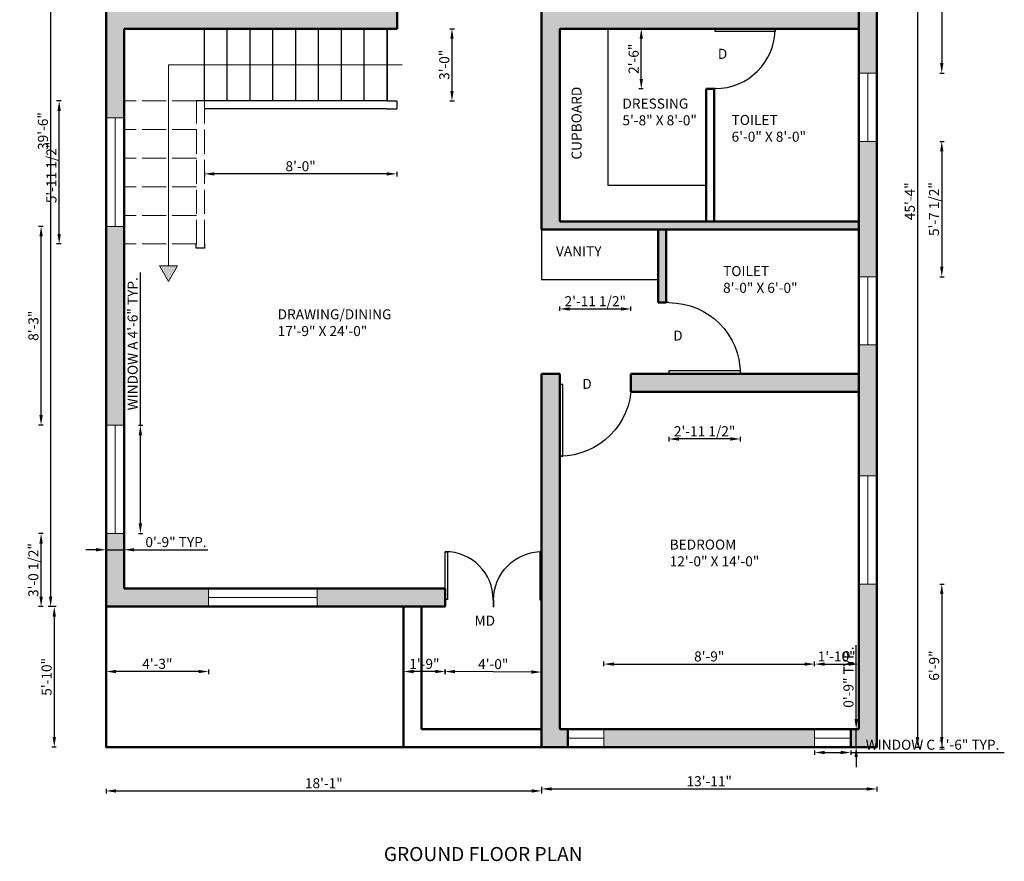
# Model space of a CAD drawing. Units: inches. Extents: x -41 to 449, y -587 to 56.
# Tile 1 of 2: x -41 to 449, y -587 to -167. Entities that reach past the tile are written whole.
import ezdxf

# ---------------------------------------------------------------- set-up
doc = ezdxf.new("R2010")
doc.units = ezdxf.units.IN
doc.linetypes.add('ACAD_ISO02W100', pattern=[15, 12, -3])
for name, color, linetype, lineweight in [('A-ANNO-DIMS', 2, 'Continuous', 18), ('A-ANNO-SYMB', 7, 'Continuous', 18), ('A-ANNO-TEXT', 7, 'Continuous', 18), ('A-ANNO-TITL', 7, 'Continuous', 35), ('A-AREA-IDEN', 7, 'Continuous', 25), ('A-DOOR', 3, 'Continuous', 25), ('A-FLOR-CASE', 8, 'Continuous', 25), ('A-FLOR-STRS', 7, 'Continuous', 25), ('A-FLOR-STRS-OVHD', 8, 'ACAD_ISO02W100', 18), ('A-GLAZ', 4, 'Continuous', 18), ('A-WALL', 7, 'Continuous', 50), ('A-WALL-PATT', 252, 'Continuous', 13)]:
    doc.layers.add(name, color=color, linetype=linetype, lineweight=lineweight)
doc.styles.get("Standard").update_dxf_attribs({"font": 'arial.ttf'})
doc.dimstyles.new('ISO-25', dxfattribs={"dimtxt": 5, "dimasz": 5, "dimexe": 1.25, "dimexo": 0.625, "dimtad": 1, "dimlunit": 3, "dimtxsty": 'Standard', "dimcen": 2.5, "dimadec": 0, "dimazin": 0, "dimtfac": 1, "dimtmove": 0, "dimatfit": 3, "dimfxl": 1, "dimfxlon": 1, "dimarcsym": 0})

# ---------------------------------------------------------------- blocks, each defined once
blk = doc.blocks.new('*U2')
for p, q in [((0, 0), (0, -6)), ((40, 0), (40, -6))]:
    blk.add_line(p, q)
blk.add_lwpolyline([(0, 0), (0, 40), (1.75, 40), (1.75, 0)], close=True)
blk.add_arc((0, 0), 40, 0, 90)
blk = doc.blocks.new('*D4')
at = {"layer": 'A-ANNO-DIMS', "color": 0, "lineweight": -2, "transparency": 16777216}
for p, q in [((404.95, 14.17), (407.2, 14.17)), ((405.95, 9.17), (405.95, -524.83)), ((404.95, -529.83), (407.2, -529.83))]:
    blk.add_line(p, q, dxfattribs=at)
at = {"layer": 'A-ANNO-DIMS', "color": 0, "transparency": 16777216}
for points in [[(405.11, 9.17), (406.78, 9.17), (405.95, 14.17)], [(405.11, -524.83), (406.78, -524.83), (405.95, -529.83)]]:
    blk.add_solid(points, dxfattribs=at)
at = {"layer": 'Defpoints', "color": 0, "transparency": 16777216}
for p in [(385.69, 14.17), (385.69, -529.83), (405.95, -529.83)]:
    blk.add_point(p, dxfattribs=at)
at = {"layer": 'A-ANNO-DIMS', "color": 0, "transparency": 16777216, "insert": (402.78, -257.83), "char_height": 5, "attachment_point": 5, "rotation": 90}
blk.add_mtext('45\'-4"', dxfattribs=at)
blk = doc.blocks.new('*D5')
at = {"layer": 'A-ANNO-DIMS', "color": 0, "lineweight": -2, "transparency": 16777216}
for p, q in [((-24.91, 14.17), (-27.16, 14.17)), ((-25.91, 9.17), (-25.91, -454.83)), ((-24.91, -459.83), (-27.16, -459.83))]:
    blk.add_line(p, q, dxfattribs=at)
at = {"layer": 'A-ANNO-DIMS', "color": 0, "transparency": 16777216}
for points in [[(-26.74, 9.17), (-25.07, 9.17), (-25.91, 14.17)], [(-26.74, -454.83), (-25.07, -454.83), (-25.91, -459.83)]]:
    blk.add_solid(points, dxfattribs=at)
at = {"layer": 'Defpoints', "color": 0, "transparency": 16777216}
for p in [(1.69, 14.17), (-25.91, -459.83), (1.69, -459.83)]:
    blk.add_point(p, dxfattribs=at)
at = {"layer": 'A-ANNO-DIMS', "color": 0, "transparency": 16777216, "insert": (-29.09, -222.83), "char_height": 5, "attachment_point": 5, "rotation": 90}
blk.add_mtext('39\'-6"', dxfattribs=at)
blk = doc.blocks.new('*D6')
at = {"layer": 'A-ANNO-DIMS', "color": 0, "lineweight": -2, "transparency": 16777216}
for p, q in [((-23.09, -459.83), (-25.34, -459.83)), ((-24.09, -464.83), (-24.09, -524.83)), ((-23.09, -529.83), (-25.34, -529.83))]:
    blk.add_line(p, q, dxfattribs=at)
at = {"layer": 'A-ANNO-DIMS', "color": 0, "transparency": 16777216}
for points in [[(-24.93, -464.83), (-23.26, -464.83), (-24.09, -459.83)], [(-24.93, -524.83), (-23.26, -524.83), (-24.09, -529.83)]]:
    blk.add_solid(points, dxfattribs=at)
at = {"layer": 'Defpoints', "color": 0, "transparency": 16777216}
for p in [(1.69, -459.83), (-24.09, -529.83), (1.69, -529.83)]:
    blk.add_point(p, dxfattribs=at)
at = {"layer": 'A-ANNO-DIMS', "color": 0, "transparency": 16777216, "insert": (-27.27, -494.83), "char_height": 5, "attachment_point": 5, "rotation": 90}
blk.add_mtext('5\'-10"', dxfattribs=at)
blk = doc.blocks.new('*D7')
at = {"layer": 'A-ANNO-DIMS', "color": 0, "lineweight": -2, "transparency": 16777216}
for p, q in [((1.69, -550.69), (1.69, -552.94)), ((6.69, -551.69), (213.69, -551.69)), ((218.69, -550.69), (218.69, -552.94))]:
    blk.add_line(p, q, dxfattribs=at)
at = {"layer": 'A-ANNO-DIMS', "color": 0, "transparency": 16777216}
for points in [[(6.69, -550.86), (6.69, -552.52), (1.69, -551.69)], [(213.69, -550.86), (213.69, -552.52), (218.69, -551.69)]]:
    blk.add_solid(points, dxfattribs=at)
at = {"layer": 'Defpoints', "color": 0, "transparency": 16777216}
for p in [(1.69, -529.83), (218.69, -529.83), (218.69, -551.69)]:
    blk.add_point(p, dxfattribs=at)
at = {"layer": 'A-ANNO-DIMS', "color": 0, "transparency": 16777216, "insert": (110.19, -548.51), "char_height": 5, "attachment_point": 5}
blk.add_mtext('18\'-1"', dxfattribs=at)
blk = doc.blocks.new('*D8')
at = {"layer": 'A-ANNO-DIMS', "color": 0, "lineweight": -2, "transparency": 16777216}
for p, q in [((218.69, -549.7), (218.69, -551.95)), ((223.69, -550.7), (380.69, -550.7)), ((385.69, -549.7), (385.69, -551.95))]:
    blk.add_line(p, q, dxfattribs=at)
at = {"layer": 'A-ANNO-DIMS', "color": 0, "transparency": 16777216}
for points in [[(223.69, -549.87), (223.69, -551.54), (218.69, -550.7)], [(380.69, -549.87), (380.69, -551.54), (385.69, -550.7)]]:
    blk.add_solid(points, dxfattribs=at)
at = {"layer": 'Defpoints', "color": 0, "transparency": 16777216}
for p in [(218.69, -529.83), (385.69, -529.83), (385.69, -550.7)]:
    blk.add_point(p, dxfattribs=at)
at = {"layer": 'A-ANNO-DIMS', "color": 0, "transparency": 16777216, "insert": (302.19, -547.52), "char_height": 5, "attachment_point": 5}
blk.add_mtext('13\'-11"', dxfattribs=at)
blk = doc.blocks.new('WIN-54IN')
blk.add_line((4.5, 54), (4.5, 0))
blk.add_lwpolyline([(0, 54), (9, 54), (9, 0), (0, 0)], close=True)
blk = doc.blocks.new('WIN-34IN')
blk.add_line((0, 4.5), (34, 4.5))
blk.add_lwpolyline([(0, 9), (34, 9), (34, 0), (0, 0)], close=True)
blk = doc.blocks.new('WIN-18IN')
blk.add_line((0, 4.5), (18, 4.5))
blk.add_lwpolyline([(0, 9), (18, 9), (18, 0), (0, 0)], close=True)
blk = doc.blocks.new('*D12')
at = {"layer": 'A-ANNO-DIMS', "color": 0, "lineweight": -2, "transparency": 16777216}
for p, q in [((18.79, -369.4), (18.79, -293.28)), ((17.79, -369.4), (20.04, -369.4)), ((18.79, -418.4), (18.79, -374.4)), ((17.79, -423.4), (20.04, -423.4))]:
    blk.add_line(p, q, dxfattribs=at)
at = {"layer": 'A-ANNO-DIMS', "color": 0, "transparency": 16777216}
for points in [[(17.96, -374.4), (19.63, -374.4), (18.79, -369.4)], [(17.96, -418.4), (19.63, -418.4), (18.79, -423.4)]]:
    blk.add_solid(points, dxfattribs=at)
at = {"layer": 'Defpoints', "color": 0, "transparency": 16777216}
for p in [(10.69, -369.4), (18.79, -369.4), (10.69, -423.4)]:
    blk.add_point(p, dxfattribs=at)
at = {"layer": 'A-ANNO-DIMS', "color": 0, "transparency": 16777216, "insert": (15.58, -328.84), "char_height": 5, "attachment_point": 5, "rotation": 90}
blk.add_mtext('WINDOW A 4\'-6" TYP.', dxfattribs=at)
blk = doc.blocks.new('*D13')
at = {"layer": 'A-ANNO-DIMS', "color": 0, "lineweight": -2, "transparency": 16777216}
for p, q in [((-3.31, -431.5), (-8.31, -431.5)), ((1.69, -430.5), (1.69, -432.75)), ((1.69, -431.5), (10.69, -431.5)), ((10.69, -430.5), (10.69, -432.75)), ((15.69, -431.5), (52.42, -431.5))]:
    blk.add_line(p, q, dxfattribs=at)
at = {"layer": 'A-ANNO-DIMS', "color": 0, "transparency": 16777216}
for points in [[(-3.31, -430.66), (-3.31, -432.33), (1.69, -431.5)], [(15.69, -430.66), (15.69, -432.33), (10.69, -431.5)]]:
    blk.add_solid(points, dxfattribs=at)
at = {"layer": 'Defpoints', "color": 0, "transparency": 16777216}
for p in [(1.69, -423.4), (10.69, -423.4), (10.69, -431.5)]:
    blk.add_point(p, dxfattribs=at)
at = {"layer": 'A-ANNO-DIMS', "color": 0, "transparency": 16777216, "insert": (36.56, -428.32), "char_height": 5, "attachment_point": 5}
blk.add_mtext('0\'-9" TYP.', dxfattribs=at)
blk = doc.blocks.new('*D16')
at = {"layer": 'A-ANNO-DIMS', "color": 0, "lineweight": -2, "transparency": 16777216}
for p, q in [((354.69, -531.53), (354.69, -533.78)), ((359.69, -532.53), (367.69, -532.53)), ((372.69, -531.53), (372.69, -533.78)), ((372.69, -532.53), (449.2, -532.53))]:
    blk.add_line(p, q, dxfattribs=at)
at = {"layer": 'A-ANNO-DIMS', "color": 0, "transparency": 16777216}
for points in [[(359.69, -531.7), (359.69, -533.37), (354.69, -532.53)], [(367.69, -531.7), (367.69, -533.37), (372.69, -532.53)]]:
    blk.add_solid(points, dxfattribs=at)
at = {"layer": 'Defpoints', "color": 0, "transparency": 16777216}
for p in [(354.69, -529.83), (372.69, -529.83), (372.69, -532.53)]:
    blk.add_point(p, dxfattribs=at)
at = {"layer": 'A-ANNO-DIMS', "color": 0, "transparency": 16777216, "insert": (413.45, -529.32), "char_height": 5, "attachment_point": 5}
blk.add_mtext('WINDOW C 1\'-6" TYP.', dxfattribs=at)
blk = doc.blocks.new('*D17')
at = {"layer": 'A-ANNO-DIMS', "color": 0, "lineweight": -2, "transparency": 16777216}
for p, q in [((375.39, -515.83), (375.39, -479.11)), ((374.39, -520.83), (376.64, -520.83)), ((375.39, -529.83), (375.39, -520.83)), ((374.39, -529.83), (376.64, -529.83)), ((375.39, -534.83), (375.39, -539.83))]:
    blk.add_line(p, q, dxfattribs=at)
at = {"layer": 'A-ANNO-DIMS', "color": 0, "transparency": 16777216}
for points in [[(374.56, -515.83), (376.23, -515.83), (375.39, -520.83)], [(374.56, -534.83), (376.23, -534.83), (375.39, -529.83)]]:
    blk.add_solid(points, dxfattribs=at)
at = {"layer": 'Defpoints', "color": 0, "transparency": 16777216}
for p in [(372.69, -520.83), (375.39, -520.83), (372.69, -529.83)]:
    blk.add_point(p, dxfattribs=at)
at = {"layer": 'A-ANNO-DIMS', "color": 0, "transparency": 16777216, "insert": (372.22, -494.97), "char_height": 5, "attachment_point": 5, "rotation": 90}
blk.add_mtext('0\'-9" TYP.', dxfattribs=at)
blk = doc.blocks.new('*D25')
at = {"layer": 'A-ANNO-DIMS', "color": 0, "lineweight": -2, "transparency": 16777216}
for p, q in [((417.04, -116.12), (419.29, -116.12)), ((418.04, -121.12), (418.04, -189)), ((417.04, -194), (419.29, -194))]:
    blk.add_line(p, q, dxfattribs=at)
at = {"layer": 'A-ANNO-DIMS', "color": 0, "transparency": 16777216}
for points in [[(417.21, -121.12), (418.88, -121.12), (418.04, -116.12)], [(417.21, -189), (418.88, -189), (418.04, -194)]]:
    blk.add_solid(points, dxfattribs=at)
at = {"layer": 'Defpoints', "color": 0, "transparency": 16777216}
for p in [(385.69, -116.12), (385.69, -194), (418.04, -194)]:
    blk.add_point(p, dxfattribs=at)
at = {"layer": 'A-ANNO-DIMS', "color": 0, "transparency": 16777216, "insert": (414.87, -155.06), "char_height": 5, "attachment_point": 5, "rotation": 90}
blk.add_mtext('6\'-6"', dxfattribs=at)
blk = doc.blocks.new('*D26')
at = {"layer": 'A-ANNO-DIMS', "color": 0, "lineweight": -2, "transparency": 16777216}
for p, q in [((417.04, -228), (419.29, -228)), ((418.04, -233), (418.04, -290.43)), ((417.04, -295.43), (419.29, -295.43))]:
    blk.add_line(p, q, dxfattribs=at)
at = {"layer": 'A-ANNO-DIMS', "color": 0, "transparency": 16777216}
for points in [[(417.21, -233), (418.88, -233), (418.04, -228)], [(417.21, -290.43), (418.88, -290.43), (418.04, -295.43)]]:
    blk.add_solid(points, dxfattribs=at)
at = {"layer": 'Defpoints', "color": 0, "transparency": 16777216}
for p in [(385.69, -228), (385.69, -295.43), (418.04, -295.43)]:
    blk.add_point(p, dxfattribs=at)
at = {"layer": 'A-ANNO-DIMS', "color": 0, "transparency": 16777216, "insert": (414.83, -261.72), "char_height": 5, "attachment_point": 5, "rotation": 90}
blk.add_mtext('5\'-7 1/2"', dxfattribs=at)
blk = doc.blocks.new('*D27')
at = {"layer": 'A-ANNO-DIMS', "color": 0, "lineweight": -2, "transparency": 16777216}
for p, q in [((417.04, -448.59), (419.29, -448.59)), ((418.04, -453.59), (418.04, -524.83)), ((417.04, -529.83), (419.29, -529.83))]:
    blk.add_line(p, q, dxfattribs=at)
at = {"layer": 'A-ANNO-DIMS', "color": 0, "transparency": 16777216}
for points in [[(417.21, -453.59), (418.88, -453.59), (418.04, -448.59)], [(417.21, -524.83), (418.88, -524.83), (418.04, -529.83)]]:
    blk.add_solid(points, dxfattribs=at)
at = {"layer": 'Defpoints', "color": 0, "transparency": 16777216}
for p in [(385.69, -448.59), (385.69, -529.83), (418.04, -529.83)]:
    blk.add_point(p, dxfattribs=at)
at = {"layer": 'A-ANNO-DIMS', "color": 0, "transparency": 16777216, "insert": (414.87, -489.21), "char_height": 5, "attachment_point": 5, "rotation": 90}
blk.add_mtext('6\'-9"', dxfattribs=at)
blk = doc.blocks.new('*D28')
at = {"layer": 'A-ANNO-DIMS', "color": 0, "lineweight": -2, "transparency": 16777216}
for p, q in [((354.69, -489.48), (354.69, -487.23)), ((359.69, -488.48), (371.69, -488.48)), ((376.69, -489.48), (376.69, -487.23))]:
    blk.add_line(p, q, dxfattribs=at)
at = {"layer": 'A-ANNO-DIMS', "color": 0, "transparency": 16777216}
for points in [[(359.69, -487.65), (359.69, -489.32), (354.69, -488.48)], [(371.69, -487.65), (371.69, -489.32), (376.69, -488.48)]]:
    blk.add_solid(points, dxfattribs=at)
at = {"layer": 'Defpoints', "color": 0, "transparency": 16777216}
for p in [(376.69, -488.48), (354.69, -520.83), (376.69, -520.83)]:
    blk.add_point(p, dxfattribs=at)
at = {"layer": 'A-ANNO-DIMS', "color": 0, "transparency": 16777216, "insert": (365.69, -485.31), "char_height": 5, "attachment_point": 5}
blk.add_mtext('1\'-10"', dxfattribs=at)
blk = doc.blocks.new('*D29')
at = {"layer": 'A-ANNO-DIMS', "color": 0, "lineweight": -2, "transparency": 16777216}
for p, q in [((249.69, -489.48), (249.69, -487.23)), ((254.69, -488.48), (349.69, -488.48)), ((354.69, -489.48), (354.69, -487.23))]:
    blk.add_line(p, q, dxfattribs=at)
at = {"layer": 'A-ANNO-DIMS', "color": 0, "transparency": 16777216}
for points in [[(254.69, -487.65), (254.69, -489.32), (249.69, -488.48)], [(349.69, -487.65), (349.69, -489.32), (354.69, -488.48)]]:
    blk.add_solid(points, dxfattribs=at)
at = {"layer": 'Defpoints', "color": 0, "transparency": 16777216}
for p in [(354.69, -488.48), (249.69, -520.83), (354.69, -520.83)]:
    blk.add_point(p, dxfattribs=at)
at = {"layer": 'A-ANNO-DIMS', "color": 0, "transparency": 16777216, "insert": (302.19, -485.31), "char_height": 5, "attachment_point": 5}
blk.add_mtext('8\'-9"', dxfattribs=at)
blk = doc.blocks.new('*D30')
at = {"layer": 'A-ANNO-DIMS', "color": 0, "lineweight": -2, "transparency": 16777216}
for p, q in [((149.87, -491.18), (149.87, -493.43)), ((165.69, -492.18), (154.87, -492.18)), ((170.69, -491.18), (170.69, -493.43))]:
    blk.add_line(p, q, dxfattribs=at)
at = {"layer": 'A-ANNO-DIMS', "color": 0, "transparency": 16777216}
for points in [[(154.87, -491.35), (154.87, -493.02), (149.87, -492.18)], [(165.69, -491.35), (165.69, -493.02), (170.69, -492.18)]]:
    blk.add_solid(points, dxfattribs=at)
at = {"layer": 'Defpoints', "color": 0, "transparency": 16777216}
for p in [(149.87, -459.83), (170.69, -459.83), (149.87, -492.18)]:
    blk.add_point(p, dxfattribs=at)
at = {"layer": 'A-ANNO-DIMS', "color": 0, "transparency": 16777216, "insert": (160.28, -489.01), "char_height": 5, "attachment_point": 5}
blk.add_mtext('1\'-9"', dxfattribs=at)
blk = doc.blocks.new('*D31')
at = {"layer": 'A-ANNO-DIMS', "color": 0, "lineweight": -2, "transparency": 16777216}
for p, q in [((170.52, -491.18), (170.51, -493.43)), ((213.62, -492.42), (175.52, -492.21)), ((218.63, -491.44), (218.62, -493.69))]:
    blk.add_line(p, q, dxfattribs=at)
at = {"layer": 'A-ANNO-DIMS', "color": 0, "transparency": 16777216}
for points in [[(175.52, -491.38), (175.51, -493.04), (170.52, -492.18)], [(213.63, -491.58), (213.62, -493.25), (218.62, -492.44)]]:
    blk.add_solid(points, dxfattribs=at)
at = {"layer": 'Defpoints', "color": 0, "transparency": 16777216}
for p in [(170.69, -459.83), (218.8, -460.09), (170.52, -492.18)]:
    blk.add_point(p, dxfattribs=at)
at = {"layer": 'A-ANNO-DIMS', "color": 0, "transparency": 16777216, "insert": (194.59, -489.14), "char_height": 5, "attachment_point": 5, "rotation": 359.6896}
blk.add_mtext('4\'-0"', dxfattribs=at)
blk = doc.blocks.new('*D32')
at = {"layer": 'A-ANNO-DIMS', "color": 0, "lineweight": -2, "transparency": 16777216}
for p, q in [((1.69, -491.18), (1.69, -493.43)), ((47.8, -492.18), (6.69, -492.18)), ((52.8, -491.18), (52.8, -493.43))]:
    blk.add_line(p, q, dxfattribs=at)
at = {"layer": 'A-ANNO-DIMS', "color": 0, "transparency": 16777216}
for points in [[(6.69, -491.35), (6.69, -493.02), (1.69, -492.18)], [(47.8, -491.35), (47.8, -493.02), (52.8, -492.18)]]:
    blk.add_solid(points, dxfattribs=at)
at = {"layer": 'Defpoints', "color": 0, "transparency": 16777216}
for p in [(1.69, -459.83), (52.8, -459.83), (1.69, -492.18)]:
    blk.add_point(p, dxfattribs=at)
at = {"layer": 'A-ANNO-DIMS', "color": 0, "transparency": 16777216, "insert": (27.25, -489), "char_height": 5, "attachment_point": 5}
blk.add_mtext('4\'-3"', dxfattribs=at)
blk = doc.blocks.new('*D33')
at = {"layer": 'A-ANNO-DIMS', "color": 0, "lineweight": -2, "transparency": 16777216}
for p, q in [((-29.66, -423.4), (-31.91, -423.4)), ((-30.66, -454.83), (-30.66, -428.4)), ((-29.66, -459.83), (-31.91, -459.83))]:
    blk.add_line(p, q, dxfattribs=at)
at = {"layer": 'A-ANNO-DIMS', "color": 0, "transparency": 16777216}
for points in [[(-31.49, -428.4), (-29.82, -428.4), (-30.66, -423.4)], [(-31.49, -454.83), (-29.82, -454.83), (-30.66, -459.83)]]:
    blk.add_solid(points, dxfattribs=at)
at = {"layer": 'Defpoints', "color": 0, "transparency": 16777216}
for p in [(-30.66, -423.4), (1.69, -423.4), (1.69, -459.83)]:
    blk.add_point(p, dxfattribs=at)
at = {"layer": 'A-ANNO-DIMS', "color": 0, "transparency": 16777216, "insert": (-33.87, -441.61), "char_height": 5, "attachment_point": 5, "rotation": 90}
blk.add_mtext('3\'-0 1/2"', dxfattribs=at)
blk = doc.blocks.new('*D34')
at = {"layer": 'A-ANNO-DIMS', "color": 0, "lineweight": -2, "transparency": 16777216}
for p, q in [((-29.66, -270.33), (-31.91, -270.33)), ((-30.66, -364.4), (-30.66, -275.33)), ((-29.66, -369.4), (-31.91, -369.4))]:
    blk.add_line(p, q, dxfattribs=at)
at = {"layer": 'A-ANNO-DIMS', "color": 0, "transparency": 16777216}
for points in [[(-31.49, -275.33), (-29.82, -275.33), (-30.66, -270.33)], [(-31.49, -364.4), (-29.82, -364.4), (-30.66, -369.4)]]:
    blk.add_solid(points, dxfattribs=at)
at = {"layer": 'Defpoints', "color": 0, "transparency": 16777216}
for p in [(-30.66, -270.33), (1.69, -270.33), (1.69, -369.4)]:
    blk.add_point(p, dxfattribs=at)
at = {"layer": 'A-ANNO-DIMS', "color": 0, "transparency": 16777216, "insert": (-33.84, -319.86), "char_height": 5, "attachment_point": 5, "rotation": 90}
blk.add_mtext('8\'-3"', dxfattribs=at)
blk = doc.blocks.new('*D37')
at = {"layer": 'A-ANNO-DIMS', "color": 0, "lineweight": -2, "transparency": 16777216}
for p, q in [((269.34, -171.83), (267.09, -171.83)), ((268.34, -196.83), (268.34, -176.83)), ((269.34, -201.83), (267.09, -201.83))]:
    blk.add_line(p, q, dxfattribs=at)
at = {"layer": 'A-ANNO-DIMS', "color": 0, "transparency": 16777216}
for points in [[(267.51, -176.83), (269.18, -176.83), (268.34, -171.83)], [(267.51, -196.83), (269.18, -196.83), (268.34, -201.83)]]:
    blk.add_solid(points, dxfattribs=at)
at = {"layer": 'Defpoints', "color": 0, "transparency": 16777216}
for p in [(268.34, -171.83), (300.69, -171.83), (300.69, -201.83)]:
    blk.add_point(p, dxfattribs=at)
at = {"layer": 'A-ANNO-DIMS', "color": 0, "transparency": 16777216, "insert": (265.17, -186.83), "char_height": 5, "attachment_point": 5, "rotation": 90}
blk.add_mtext('2\'-6"', dxfattribs=at)
blk = doc.blocks.new('*D38')
at = {"layer": 'A-ANNO-DIMS', "color": 0, "lineweight": -2, "transparency": 16777216}
for p, q in [((282.11, -375.29), (282.11, -377.54)), ((312.69, -376.29), (287.11, -376.29)), ((317.69, -375.29), (317.69, -377.54))]:
    blk.add_line(p, q, dxfattribs=at)
at = {"layer": 'A-ANNO-DIMS', "color": 0, "transparency": 16777216}
for points in [[(287.11, -375.45), (287.11, -377.12), (282.11, -376.29)], [(312.69, -375.45), (312.69, -377.12), (317.69, -376.29)]]:
    blk.add_solid(points, dxfattribs=at)
at = {"layer": 'Defpoints', "color": 0, "transparency": 16777216}
for p in [(282.11, -343.94), (317.69, -343.94), (282.11, -376.29)]:
    blk.add_point(p, dxfattribs=at)
at = {"layer": 'A-ANNO-DIMS', "color": 0, "transparency": 16777216, "insert": (299.9, -373.08), "char_height": 5, "attachment_point": 5}
blk.add_mtext('2\'-11 1/2"', dxfattribs=at)
blk = doc.blocks.new('*D39')
at = {"layer": 'A-ANNO-DIMS', "color": 0, "lineweight": -2, "transparency": 16777216}
for p, q in [((227.69, -312.48), (227.69, -310.23)), ((232.69, -311.48), (258.19, -311.48)), ((263.19, -312.48), (263.19, -310.23))]:
    blk.add_line(p, q, dxfattribs=at)
at = {"layer": 'A-ANNO-DIMS', "color": 0, "transparency": 16777216}
for points in [[(232.69, -310.65), (232.69, -312.32), (227.69, -311.48)], [(258.19, -310.65), (258.19, -312.32), (263.19, -311.48)]]:
    blk.add_solid(points, dxfattribs=at)
at = {"layer": 'Defpoints', "color": 0, "transparency": 16777216}
for p in [(263.19, -311.48), (227.69, -343.83), (263.19, -343.83)]:
    blk.add_point(p, dxfattribs=at)
at = {"layer": 'A-ANNO-DIMS', "color": 0, "transparency": 16777216, "insert": (245.44, -308.27), "char_height": 5, "attachment_point": 5}
blk.add_mtext('2\'-11 1/2"', dxfattribs=at)
blk = doc.blocks.new('*D40')
at = {"layer": 'A-ANNO-DIMS', "color": 0, "lineweight": -2, "transparency": 16777216}
for p, q in [((173.02, -171.83), (175.27, -171.83)), ((174.02, -176.83), (174.02, -202.83)), ((173.02, -207.83), (175.27, -207.83))]:
    blk.add_line(p, q, dxfattribs=at)
at = {"layer": 'A-ANNO-DIMS', "color": 0, "transparency": 16777216}
for points in [[(173.19, -176.83), (174.86, -176.83), (174.02, -171.83)], [(173.19, -202.83), (174.86, -202.83), (174.02, -207.83)]]:
    blk.add_solid(points, dxfattribs=at)
at = {"layer": 'Defpoints', "color": 0, "transparency": 16777216}
for p in [(141.67, -171.83), (141.67, -207.83), (174.02, -207.83)]:
    blk.add_point(p, dxfattribs=at)
at = {"layer": 'A-ANNO-DIMS', "color": 0, "transparency": 16777216, "insert": (170.84, -189.83), "char_height": 5, "attachment_point": 5, "rotation": 90}
blk.add_mtext('3\'-0"', dxfattribs=at)
blk = doc.blocks.new('*D41')
at = {"layer": 'A-ANNO-DIMS', "color": 0, "lineweight": -2, "transparency": 16777216}
for p, q in [((50.69, -243.18), (50.69, -245.43)), ((141.54, -244.18), (55.69, -244.18)), ((146.54, -243.18), (146.54, -245.43))]:
    blk.add_line(p, q, dxfattribs=at)
at = {"layer": 'A-ANNO-DIMS', "color": 0, "transparency": 16777216}
for points in [[(55.69, -243.35), (55.69, -245.02), (50.69, -244.18)], [(141.54, -243.35), (141.54, -245.02), (146.54, -244.18)]]:
    blk.add_solid(points, dxfattribs=at)
at = {"layer": 'Defpoints', "color": 0, "transparency": 16777216}
for p in [(50.69, -211.83), (146.54, -211.83), (50.69, -244.18)]:
    blk.add_point(p, dxfattribs=at)
at = {"layer": 'A-ANNO-DIMS', "color": 0, "transparency": 16777216, "insert": (98.62, -241.01), "char_height": 5, "attachment_point": 5}
blk.add_mtext('8\'-0"', dxfattribs=at)
blk = doc.blocks.new('*D42')
at = {"layer": 'A-ANNO-DIMS', "color": 0, "lineweight": -2, "transparency": 16777216}
for p, q in [((-20.66, -207.83), (-22.91, -207.83)), ((-21.66, -274.12), (-21.66, -212.83)), ((-20.66, -279.12), (-22.91, -279.12))]:
    blk.add_line(p, q, dxfattribs=at)
at = {"layer": 'A-ANNO-DIMS', "color": 0, "transparency": 16777216}
for points in [[(-22.49, -212.83), (-20.82, -212.83), (-21.66, -207.83)], [(-22.49, -274.12), (-20.82, -274.12), (-21.66, -279.12)]]:
    blk.add_solid(points, dxfattribs=at)
at = {"layer": 'Defpoints', "color": 0, "transparency": 16777216}
for p in [(-21.66, -207.83), (10.69, -207.83), (10.69, -279.12)]:
    blk.add_point(p, dxfattribs=at)
at = {"layer": 'A-ANNO-DIMS', "color": 0, "transparency": 16777216, "insert": (-24.87, -243.48), "char_height": 5, "attachment_point": 5, "rotation": 90}
blk.add_mtext('5\'-11 1/2"', dxfattribs=at)

msp = doc.modelspace()

# ---------------------------------------------------------------- hatches: boundary and pattern name
at = {"layer": 'A-ANNO-SYMB'}
h = msp.add_hatch(color=256, dxfattribs=at)
h.dxf.hatch_style = 1
h.paths.add_polyline_path([(32.828, -297.816), (37.328, -290.021), (28.328, -290.021)])
at = {"layer": 'A-WALL-PATT'}
h = msp.add_hatch(color=256, dxfattribs=at)
h.dxf.hatch_style = 1
h.paths.add_polyline_path([(106.669, 14.166), (65.62, 14.166), (65.62, 5.166), (106.695, 5.166), (106.695, 7.401, -0.0094448), (106.669, 8.762)], flags=17)
h.paths.add_polyline_path([(31.62, 14.166), (1.695, 14.166), (1.695, -216.327), (10.695, -216.327), (10.695, -171.834), (146.695, -171.834), (146.695, -162.834), (10.695, -162.834), (10.695, 5.166), (31.62, 5.166)])
h.paths.add_polyline_path([(167.994, 14.166), (142.695, 14.166), (142.695, 8.762), (142.695, -27.264), (142.695, -90.806), (146.695, -90.806), (146.695, 5.166), (167.994, 5.166)])
h.paths.add_polyline_path([(232.757, 14.166), (201.994, 14.166), (201.994, 5.166), (218.695, 5.166), (218.695, -120.834), (142.695, -120.834), (142.695, -124.834), (146.695, -124.834), (218.695, -124.834), (227.695, -124.834), (227.695, 5.166), (232.757, 5.166)])
h.paths.add_polyline_path([(350.174, 14.166), (250.757, 14.166), (250.757, 5.166), (350.174, 5.166)])
h.paths.add_polyline_path([(385.695, 14.166), (368.174, 14.166), (368.174, 5.166), (376.695, 5.166), (376.695, -62.119), (385.695, -62.119)])
h.paths.add_polyline_path([(385.695, -116.119), (376.695, -116.119), (376.695, -194.002), (385.695, -194.002)])
h.paths.add_polyline_path([(376.695, -162.834), (227.695, -162.834), (224.376, -162.834), (218.695, -162.834), (218.695, -271.834), (227.695, -271.834), (376.695, -271.834), (376.695, -267.834), (227.695, -267.834), (227.695, -171.834), (376.695, -171.834)])
h.paths.add_polyline_path([(385.695, -228.002), (376.695, -228.002), (376.695, -295.429), (385.695, -295.429)])
h.paths.add_polyline_path([(385.695, -329.429), (376.695, -329.429), (376.695, -394.588), (385.695, -394.588)])
h.paths.add_polyline_path([(376.695, -343.834), (317.695, -343.834), (317.695, -343.936), (282.107, -343.936), (276.769, -343.936), (263.368, -343.835), (263.368, -349.185, -0.0248206), (263.192, -352.72), (263.192, -352.834), (376.695, -352.834)])
h.paths.add_polyline_path([(280.695, -271.834), (276.695, -271.834), (276.695, -308.243), (280.695, -308.243)])
h.paths.add_polyline_path([(227.695, -343.834), (218.695, -343.834), (218.695, -432.415), (218.799, -432.415), (218.799, -456.484), (218.799, -460.095), (218.695, -520.834), (218.695, -529.834), (231.695, -529.834), (231.695, -520.834), (227.695, -520.834)])
h.paths.add_polyline_path([(354.695, -520.834), (249.695, -520.834), (249.695, -529.834), (354.695, -529.834)])
h.paths.add_polyline_path([(385.695, -448.588), (376.695, -448.588), (376.695, -520.834), (372.695, -520.834), (372.695, -529.834), (385.695, -529.834)])
h.paths.add_polyline_path([(170.695, -456.353), (170.695, -450.834), (106.802, -450.834), (106.802, -459.834), (170.695, -459.834)])
h.paths.add_polyline_path([(52.802, -450.834), (10.695, -450.834), (10.695, -423.396), (1.695, -423.396), (1.695, -459.834), (52.802, -459.834)])
h.paths.add_polyline_path([(10.695, -270.327), (1.695, -270.327), (1.695, -369.396), (10.695, -369.396)])

# ---------------------------------------------------------------- linework, layer by layer
at = {"layer": 'A-ANNO-SYMB'}
for p, q in [((141.672, -189.834), (32.828, -189.834)), ((32.828, -189.834), (32.828, -290.021)), ((141.672, -189.834), (149.193, -189.834)), ((37.328, -290.021), (28.328, -290.021)), ((28.328, -290.021), (32.828, -297.816)), ((32.828, -297.816), (37.328, -290.021))]:
    msp.add_line(p, q, dxfattribs=at)
at = {"layer": 'A-FLOR-CASE'}
for p, q in [((251.695, -171.834), (251.695, -249.721)), ((251.695, -249.721), (300.695, -249.721)), ((218.695, -271.834), (218.695, -296.833)), ((218.695, -296.833), (276.695, -296.833))]:
    msp.add_line(p, q, dxfattribs=at)
at = {"layer": 'A-FLOR-STRS'}
for p, q in [((50.695, -207.834), (50.695, -171.834)), ((62.067, -207.834), (62.067, -171.834)), ((73.439, -207.834), (73.439, -171.834)), ((84.811, -207.834), (84.811, -171.834)), ((96.183, -207.834), (96.183, -171.834)), ((107.555, -207.834), (107.555, -171.834)), ((118.928, -207.834), (118.928, -171.834)), ((130.3, -207.834), (130.3, -171.834)), ((141.672, -171.834), (141.672, -207.834)), ((141.672, -207.834), (141.672, -171.834)), ((50.695, -207.834), (46.695, -207.834)), ((141.672, -207.834), (50.695, -207.834)), ((141.672, -207.834), (146.542, -207.834)), ((146.542, -207.834), (146.542, -211.834)), ((141.672, -211.834), (50.695, -211.834)), ((141.672, -211.834), (146.542, -211.834)), ((46.672, -281.229), (46.672, -279.116)), ((50.695, -279.116), (50.695, -281.229)), ((50.695, -281.229), (46.672, -281.229))]:
    msp.add_line(p, q, dxfattribs=at)
at = {"layer": 'A-FLOR-STRS-OVHD'}
for p, q in [((46.695, -207.834), (10.695, -207.834)), ((46.695, -279.116), (46.695, -207.834)), ((50.695, -279.116), (50.695, -207.834)), ((46.695, -222.09), (10.695, -222.09)), ((46.695, -236.347), (10.695, -236.347)), ((46.695, -250.603), (10.695, -250.603)), ((46.695, -264.86), (10.695, -264.86)), ((46.695, -279.116), (10.695, -279.116)), ((46.695, -279.116), (10.695, -279.116))]:
    msp.add_line(p, q, dxfattribs=at)
at = {"layer": 'A-WALL'}
for p, q in [((376.695, 5.166), (376.695, -520.834)), ((146.695, -171.834), (146.695, -162.834)), ((218.695, -271.834), (218.695, -162.834)), ((10.695, -171.834), (146.695, -171.834)), ((10.695, -450.834), (10.695, -171.834)), ((227.695, -171.834), (376.695, -171.834)), ((227.695, -267.834), (227.695, -171.834)), ((300.695, -267.834), (300.695, -201.834)), ((304.695, -201.834), (300.695, -201.834)), ((304.695, -267.834), (304.695, -201.834)), ((227.695, -267.834), (376.695, -267.834)), ((227.695, -271.834), (218.695, -271.834)), ((227.695, -271.834), (376.695, -271.834)), ((276.695, -271.834), (276.695, -308.243)), ((280.695, -271.834), (280.695, -308.243)), ((280.695, -308.243), (276.695, -308.243)), ((218.695, -520.834), (218.695, -343.834)), ((227.695, -343.834), (218.695, -343.834)), ((227.695, -520.834), (227.695, -343.834)), ((263.192, -343.834), (376.695, -343.834)), ((263.192, -352.834), (263.192, -343.834)), ((263.192, -352.834), (376.695, -352.834)), ((170.695, -450.834), (10.695, -450.834)), ((170.695, -459.834), (170.695, -450.834)), ((170.695, -459.834), (1.695, -459.834)), ((149.866, -529.834), (149.866, -459.834)), ((158.866, -520.834), (158.866, -459.834)), ((218.695, -520.834), (158.866, -520.834)), ((218.695, -520.834), (218.695, -529.834)), ((376.695, -520.834), (227.695, -520.834)), ((231.695, -520.834), (231.695, -529.834)), ((372.695, -520.834), (372.695, -529.834))]:
    msp.add_line(p, q, dxfattribs=at)
msp.add_lwpolyline([(142.695, 14.166), (385.695, 14.166), (385.695, -529.834), (1.695, -529.834), (1.695, 14.166), (106.695, 14.166)], dxfattribs=at)

# ---------------------------------------------------------------- block references
at = {"layer": 'A-DOOR'}
for p, xscale, yscale, zscale, rotation in [((305.172, -171.834), 0.7463213848148805, 0.7463213848148805, 0.7463213848148805, 270), ((282.107, -343.936), -0.8896844596356588, 0.8896844596356588, 0.8896844596356588, 270), ((227.695, -349.185), -0.8918248732798799, 0.8918248732798799, 0.8918248732798799, 180)]:
    msp.add_blockref('*U2', p, dxfattribs=dict(at, xscale=xscale, yscale=yscale, zscale=zscale, rotation=rotation))
for p, xscale, yscale, zscale in [((170.695, -456.353), 0.5973605819935102, 0.5973605819935102, 0.5973605819935102), ((218.799, -456.484), -0.6017225957490285, 0.6017225957490285, 0.6017225957490285)]:
    msp.add_blockref('*U2', p, dxfattribs=dict(at, xscale=xscale, yscale=yscale, zscale=zscale))
at = {"layer": 'A-GLAZ', "rotation": 269.9999999999999}
for name, p in [('WIN-34IN', (376.695, -194.002)), ('WIN-34IN', (376.695, -295.429)), ('WIN-54IN', (52.802, -450.834))]:
    msp.add_blockref(name, p, dxfattribs=at)
at = {"layer": 'A-GLAZ'}
for name, p in [('WIN-54IN', (1.695, -270.327)), ('WIN-54IN', (1.695, -423.396)), ('WIN-54IN', (376.695, -448.588)), ('WIN-18IN', (231.695, -529.834)), ('WIN-18IN', (354.695, -529.834))]:
    msp.add_blockref(name, p, dxfattribs=at)

# ---------------------------------------------------------------- texts
at = {"layer": 'A-ANNO-TEXT', "char_height": 5, "attachment_point": 1}
for s, width, insert in [('D', 11.20392, (306.491, -181.858)), ('VANITY', 33.10657, (225.841, -280.216)), ('D', 11.47104, (284.257, -322.251)), ('D', 13.47847, (238.946, -346.321)), ('MD', 2.74804, (185.277, -464.327))]:
    msp.add_mtext_dynamic_manual_height_columns(s, width=width, gutter_width=12.5, heights=[0], dxfattribs=dict(at, insert=insert))
at = {"layer": 'A-ANNO-TEXT', "insert": (233.59, -237.051), "char_height": 5, "attachment_point": 1, "rotation": 90}
msp.add_mtext_dynamic_manual_height_columns('CUPBOARD', width=59.17481, gutter_width=12.5, heights=[0], dxfattribs=at)
at = {"layer": 'A-ANNO-TITL', "insert": (140.084, -579.641), "char_height": 7, "attachment_point": 1}
msp.add_mtext_dynamic_manual_height_columns('GROUND FLOOR PLAN', width=251.13092, gutter_width=12.5, heights=[0], dxfattribs=at)
at = {"layer": 'A-AREA-IDEN', "char_height": 5, "attachment_point": 1}
for s, width, insert in [('DRESSING\\P5\'-8" X 8\'-0"', 46.49449, (258.951, -206.642)), ('TOILET\\P6\'-0" X 8\'-0"', 54.94804, (313.335, -214.807)), ('TOILET\\P8\'-0" X 6\'-0"', 53.64831, (309.101, -290.133)), ('DRAWING/DINING\\P17\'-9" X 24\'-0"', 106.1228, (87.179, -311.67)), ('BEDROOM\\P12\'-0" X 14\'-0"', 91.67854, (282.486, -426.428))]:
    msp.add_mtext_dynamic_manual_height_columns(s, width=width, gutter_width=12.5, heights=[0], dxfattribs=dict(at, insert=insert))

# ---------------------------------------------------------------- dimensions: what is measured, and where the dimension line sits
at = {"layer": 'A-ANNO-DIMS'}
for base, p1, p2, angle, override, picture, middle in [((-25.907, -459.834), (1.695, 14.166), (1.695, -459.834), 90, {"dimclrd": 0, "dimclre": 0, "dimclrt": 0}, '*D5', (-29.087, -222.834)), ((405.948, -529.834), (385.695, 14.166), (385.695, -529.834), 90, {"dimclrd": 0, "dimclre": 0, "dimclrt": 0}, '*D4', (402.781, -257.834)), ((418.045, -194.002), (385.695, -116.119), (385.695, -194.002), 270, {"dimdec": 1, "dimlfac": 1, "dimrnd": 0, "dimzin": 1, "dimdsep": 46, "dimlunit": 4, "dimfrac": 2}, '*D25', (414.867, -155.06)), ((174.022, -207.834), (141.672, -171.834), (141.672, -207.834), 270, {"dimdec": 1, "dimlfac": 1, "dimrnd": 0, "dimzin": 1, "dimdsep": 46, "dimlunit": 4, "dimfrac": 2}, '*D40', (170.842, -189.834)), ((268.345, -171.834), (300.695, -201.834), (300.695, -171.834), 90, {"dimdec": 1, "dimlfac": 1, "dimrnd": 0, "dimzin": 1, "dimdsep": 46, "dimlunit": 4, "dimfrac": 2}, '*D37', (265.167, -186.834)), ((-21.655, -207.834), (10.695, -279.116), (10.695, -207.834), 90, {"dimdec": 1, "dimlfac": 1, "dimrnd": 0, "dimzin": 1, "dimdsep": 46, "dimlunit": 4, "dimfrac": 2}, '*D42', (-24.866, -243.475)), ((50.695, -244.184), (146.542, -211.834), (50.695, -211.834), 180, {"dimdec": 1, "dimlfac": 1, "dimrnd": 0, "dimzin": 1, "dimdsep": 46, "dimlunit": 4, "dimfrac": 2}, '*D41', (98.618, -241.006)), ((418.045, -295.429), (385.695, -228.002), (385.695, -295.429), 270, {"dimdec": 1, "dimlfac": 1, "dimrnd": 0, "dimzin": 1, "dimdsep": 46, "dimlunit": 4, "dimfrac": 2}, '*D26', (414.834, -261.715)), ((-30.655, -270.327), (1.695, -369.396), (1.695, -270.327), 90, {"dimdec": 1, "dimlfac": 1, "dimrnd": 0, "dimzin": 1, "dimdsep": 46, "dimlunit": 4, "dimfrac": 2}, '*D34', (-33.835, -319.861)), ((282.107, -376.286), (317.695, -343.936), (282.107, -343.936), 180, {"dimdec": 1, "dimlfac": 1, "dimrnd": 0, "dimzin": 1, "dimdsep": 46, "dimlunit": 4, "dimfrac": 2}, '*D38', (299.901, -373.076)), ((-30.655, -423.396), (1.695, -459.834), (1.695, -423.396), 90, {"dimdec": 1, "dimlfac": 1, "dimrnd": 0, "dimzin": 1, "dimdsep": 46, "dimlunit": 4, "dimfrac": 2}, '*D33', (-33.867, -441.615)), ((418.045, -529.834), (385.695, -448.588), (385.695, -529.834), 270, {"dimdec": 1, "dimlfac": 1, "dimrnd": 0, "dimzin": 1, "dimdsep": 46, "dimlunit": 4, "dimfrac": 2}, '*D27', (414.867, -489.211)), ((-24.094, -529.834), (1.695, -459.834), (1.695, -529.834), 90, {"dimclrd": 0, "dimclre": 0, "dimclrt": 0}, '*D6', (-27.272, -494.834)), ((1.695, -492.184), (52.802, -459.834), (1.695, -459.834), 180, {"dimdec": 1, "dimlfac": 1, "dimrnd": 0, "dimzin": 1, "dimdsep": 46, "dimlunit": 4, "dimfrac": 2}, '*D32', (27.248, -489.004)), ((149.866, -492.184), (170.695, -459.834), (149.866, -459.834), 180, {"dimdec": 1, "dimlfac": 1, "dimrnd": 0, "dimzin": 1, "dimdsep": 46, "dimlunit": 4, "dimfrac": 2}, '*D30', (160.281, -489.006)), ((170.519, -492.184), (218.799, -460.095), (170.695, -459.834), 179.6896, {"dimdec": 1, "dimlfac": 1, "dimrnd": 0, "dimzin": 1, "dimdsep": 46, "dimlunit": 4, "dimfrac": 2}, '*D31', (194.589, -489.136)), ((376.695, -488.484), (354.695, -520.834), (376.695, -520.834), 0, {"dimdec": 1, "dimlfac": 1, "dimrnd": 0, "dimzin": 1, "dimdsep": 46, "dimlunit": 4, "dimfrac": 2}, '*D28', (365.695, -485.306))]:
    dim = msp.add_linear_dim(base=base, p1=p1, p2=p2, angle=angle, dimstyle='ISO-25', override=override, dxfattribs=at)
    dim.commit()
    dim.dimension.update_dxf_attribs({"geometry": picture, "text_midpoint": middle})
for base, p1, p2, text, picture, middle in [((18.795, -369.396), (10.695, -423.396), (10.695, -369.396), 'WINDOW A <> TYP.', '*D12', (15.583, -328.835)), ((375.395, -520.834), (372.695, -529.834), (372.695, -520.834), '<> TYP.', '*D17', (372.217, -494.97))]:
    dim = msp.add_linear_dim(base=base, p1=p1, p2=p2, angle=90, text=text, dimstyle='ISO-25', override={"dimdec": 1, "dimlfac": 1, "dimrnd": 0, "dimzin": 1, "dimdsep": 46, "dimlunit": 4, "dimfrac": 2}, dxfattribs=at)
    dim.commit()
    dim.dimension.update_dxf_attribs({"geometry": picture, "text_midpoint": middle})
for base, p1, p2, override, picture, middle in [((263.192, -311.484), (227.695, -343.834), (263.192, -343.834), {"dimdec": 1, "dimlfac": 1, "dimrnd": 0, "dimzin": 1, "dimdsep": 46, "dimlunit": 4, "dimfrac": 2}, '*D39', (245.443, -308.274)), ((354.695, -488.484), (249.695, -520.834), (354.695, -520.834), {"dimdec": 1, "dimlfac": 1, "dimrnd": 0, "dimzin": 1, "dimdsep": 46, "dimlunit": 4, "dimfrac": 2}, '*D29', (302.195, -485.306)), ((218.695, -551.691), (1.695, -529.834), (218.695, -529.834), {"dimclrd": 0, "dimclre": 0, "dimclrt": 0}, '*D7', (110.195, -548.513)), ((385.695, -550.703), (218.695, -529.834), (385.695, -529.834), {"dimclrd": 0, "dimclre": 0, "dimclrt": 0}, '*D8', (302.195, -547.523))]:
    dim = msp.add_linear_dim(base=base, p1=p1, p2=p2, dimstyle='ISO-25', override=override, dxfattribs=at)
    dim.commit()
    dim.dimension.update_dxf_attribs({"geometry": picture, "text_midpoint": middle})
for base, p1, p2, text, picture, middle in [((10.695, -431.496), (1.695, -423.396), (10.695, -423.396), '<> TYP.', '*D13', (36.558, -428.318)), ((372.695, -532.534), (354.695, -529.834), (372.695, -529.834), 'WINDOW C <> TYP.', '*D16', (413.447, -529.322))]:
    dim = msp.add_linear_dim(base=base, p1=p1, p2=p2, text=text, dimstyle='ISO-25', override={"dimdec": 1, "dimlfac": 1, "dimrnd": 0, "dimzin": 1, "dimdsep": 46, "dimlunit": 4, "dimfrac": 2}, dxfattribs=at)
    dim.commit()
    dim.dimension.update_dxf_attribs({"geometry": picture, "text_midpoint": middle})

doc.saveas('drawing.dxf')
